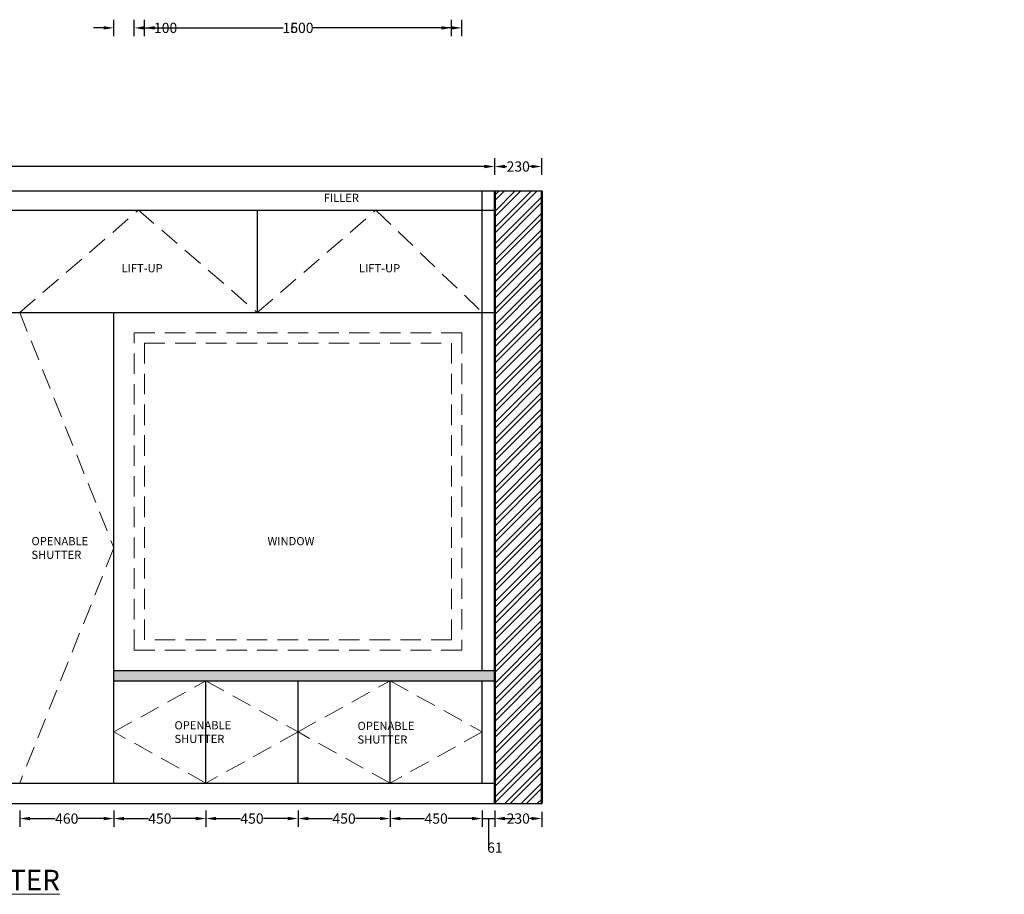
# Model space of a CAD drawing. Units: millimetres. Extents: x -472 to 16192, y -4730 to 4331.
# Tile 2 of 8: x 3049 to 7860, y -4730 to -455. Entities that reach past the tile are written whole.
import ezdxf

# ---------------------------------------------------------------- set-up
doc = ezdxf.new("R2010")
doc.units = ezdxf.units.MM
doc.header["$MEASUREMENT"] = 0
doc.linetypes.add('DASHED', pattern=[0.75, 0.5, -0.25])
for name, color, linetype, lineweight in [('A-ANNO-DIMS', 2, 'Continuous', 18), ('A-ANNO-TEXT', 6, 'Continuous', 18), ('A-ELEV', 7, 'Continuous', 25), ('A-ELEV-SWNG', 4, 'DASHED', 13), ('A-GLAZ', 4, 'DASHED', 18), ('A-WALL', 7, 'Continuous', 50), ('A-WALL-PATT', 8, 'Continuous', 13)]:
    doc.layers.add(name, color=color, linetype=linetype, lineweight=lineweight)
doc.styles.get("Standard").update_dxf_attribs({"font": 'arial.ttf'})
doc.dimstyles.get("Standard").update_dxf_attribs({"dimtxt": 50, "dimasz": 50, "dimexe": 40, "dimexo": 40, "dimgap": 0.09, "dimtad": 0, "dimtih": 1, "dimtoh": 1, "dimdec": 0, "dimzin": 0, "dimdsep": 46, "dimtxsty": 'Standard', "dimcen": 0.09, "dimclrd": 1, "dimclre": 3, "dimclrt": 6, "dimadec": 0, "dimazin": 0, "dimtfac": 1, "dimtdec": 0, "dimtofl": 0, "dimtmove": 0, "dimatfit": 3, "dimfxl": 40, "dimfxlon": 1, "dimtolj": 1, "dimtzin": 0, "dimarcsym": 0})

# ---------------------------------------------------------------- blocks, each defined once
blk = doc.blocks.new('*D17')
at = {"layer": 'A-ANNO-DIMS', "color": 0, "lineweight": -2, "transparency": 16777216}
for p, q in [((230, -1212.4), (230, -1132.4)), ((5370, -1212.4), (5370, -1132.4)), ((280, -1172.4), (2725.3, -1172.4)), ((5320, -1172.4), (2874.7, -1172.4))]:
    blk.add_line(p, q, dxfattribs=at)
at = {"layer": 'A-ANNO-DIMS', "color": 0, "transparency": 16777216}
for points in [[(280, -1164.1), (280, -1180.8), (230, -1172.4)], [(5320, -1164.1), (5320, -1180.8), (5370, -1172.4)]]:
    blk.add_solid(points, dxfattribs=at)
at = {"layer": 'Defpoints', "color": 0, "transparency": 16777216}
for p in [(5370, -1172.4), (230, -1290.9), (5370, -1290.9)]:
    blk.add_point(p, dxfattribs=at)
at = {"layer": 'A-ANNO-DIMS', "color": 0, "transparency": 16777216, "insert": (2800, -1172.4), "char_height": 50, "attachment_point": 5}
blk.add_mtext('\\A1;5140', dxfattribs=at)
blk = doc.blocks.new('*D18')
at = {"layer": 'A-ANNO-DIMS', "color": 0, "lineweight": -2, "transparency": 16777216}
for p, q in [((5370, -1212.4), (5370, -1132.4)), ((5600, -1212.4), (5600, -1132.4)), ((5420, -1172.4), (5429.3, -1172.4)), ((5550, -1172.4), (5540.7, -1172.4))]:
    blk.add_line(p, q, dxfattribs=at)
at = {"layer": 'A-ANNO-DIMS', "color": 0, "transparency": 16777216}
for points in [[(5420, -1164.1), (5420, -1180.8), (5370, -1172.4)], [(5550, -1164.1), (5550, -1180.8), (5600, -1172.4)]]:
    blk.add_solid(points, dxfattribs=at)
at = {"layer": 'Defpoints', "color": 0, "transparency": 16777216}
for p in [(5600, -1172.4), (5370, -1290.9), (5600, -1290.9)]:
    blk.add_point(p, dxfattribs=at)
at = {"layer": 'A-ANNO-DIMS', "color": 0, "transparency": 16777216, "insert": (5485, -1172.4), "char_height": 50, "attachment_point": 5}
blk.add_mtext('\\A1;230', dxfattribs=at)
blk = doc.blocks.new('*D34')
at = {"layer": 'A-ANNO-DIMS', "color": 0, "lineweight": -2, "transparency": 16777216}
for p, q in [((3049, -4319.4), (3049, -4399.4)), ((3509, -4319.4), (3509, -4399.4)), ((3099, -4359.4), (3222.8, -4359.4)), ((3459, -4359.4), (3335.2, -4359.4))]:
    blk.add_line(p, q, dxfattribs=at)
at = {"layer": 'A-ANNO-DIMS', "color": 0, "transparency": 16777216}
for points in [[(3099, -4351), (3099, -4367.7), (3049, -4359.4)], [(3459, -4351), (3459, -4367.7), (3509, -4359.4)]]:
    blk.add_solid(points, dxfattribs=at)
at = {"layer": 'Defpoints', "color": 0, "transparency": 16777216}
for p in [(3049, -4185.9), (3509, -4185.9), (3509, -4359.4)]:
    blk.add_point(p, dxfattribs=at)
at = {"layer": 'A-ANNO-DIMS', "color": 0, "transparency": 16777216, "insert": (3279, -4359.4), "char_height": 50, "attachment_point": 5}
blk.add_mtext('\\A1;460', dxfattribs=at)
blk = doc.blocks.new('*D35')
at = {"layer": 'A-ANNO-DIMS', "color": 0, "lineweight": -2, "transparency": 16777216}
for p, q in [((3509, -4319.4), (3509, -4399.4)), ((3959, -4319.4), (3959, -4399.4)), ((3559, -4359.4), (3677.8, -4359.4)), ((3909, -4359.4), (3790.2, -4359.4))]:
    blk.add_line(p, q, dxfattribs=at)
at = {"layer": 'A-ANNO-DIMS', "color": 0, "transparency": 16777216}
for points in [[(3559, -4351), (3559, -4367.7), (3509, -4359.4)], [(3909, -4351), (3909, -4367.7), (3959, -4359.4)]]:
    blk.add_solid(points, dxfattribs=at)
at = {"layer": 'Defpoints', "color": 0, "transparency": 16777216}
for p in [(3509, -4185.9), (3959, -4185.9), (3959, -4359.4)]:
    blk.add_point(p, dxfattribs=at)
at = {"layer": 'A-ANNO-DIMS', "color": 0, "transparency": 16777216, "insert": (3734, -4359.4), "char_height": 50, "attachment_point": 5}
blk.add_mtext('\\A1;450', dxfattribs=at)
blk = doc.blocks.new('*D36')
at = {"layer": 'A-ANNO-DIMS', "color": 0, "lineweight": -2, "transparency": 16777216}
for p, q in [((3959, -4319.4), (3959, -4399.4)), ((4409, -4319.4), (4409, -4399.4)), ((4009, -4359.4), (4127.8, -4359.4)), ((4359, -4359.4), (4240.2, -4359.4))]:
    blk.add_line(p, q, dxfattribs=at)
at = {"layer": 'A-ANNO-DIMS', "color": 0, "transparency": 16777216}
for points in [[(4009, -4351), (4009, -4367.7), (3959, -4359.4)], [(4359, -4351), (4359, -4367.7), (4409, -4359.4)]]:
    blk.add_solid(points, dxfattribs=at)
at = {"layer": 'Defpoints', "color": 0, "transparency": 16777216}
for p in [(3959, -4185.9), (4409, -4185.9), (4409, -4359.4)]:
    blk.add_point(p, dxfattribs=at)
at = {"layer": 'A-ANNO-DIMS', "color": 0, "transparency": 16777216, "insert": (4184, -4359.4), "char_height": 50, "attachment_point": 5}
blk.add_mtext('\\A1;450', dxfattribs=at)
blk = doc.blocks.new('*D37')
at = {"layer": 'A-ANNO-DIMS', "color": 0, "lineweight": -2, "transparency": 16777216}
for p, q in [((4409, -4319.4), (4409, -4399.4)), ((4859, -4319.4), (4859, -4399.4)), ((4459, -4359.4), (4577.8, -4359.4)), ((4809, -4359.4), (4690.2, -4359.4))]:
    blk.add_line(p, q, dxfattribs=at)
at = {"layer": 'A-ANNO-DIMS', "color": 0, "transparency": 16777216}
for points in [[(4459, -4351), (4459, -4367.7), (4409, -4359.4)], [(4809, -4351), (4809, -4367.7), (4859, -4359.4)]]:
    blk.add_solid(points, dxfattribs=at)
at = {"layer": 'Defpoints', "color": 0, "transparency": 16777216}
for p in [(4409, -4185.9), (4859, -4185.9), (4859, -4359.4)]:
    blk.add_point(p, dxfattribs=at)
at = {"layer": 'A-ANNO-DIMS', "color": 0, "transparency": 16777216, "insert": (4634, -4359.4), "char_height": 50, "attachment_point": 5}
blk.add_mtext('\\A1;450', dxfattribs=at)
blk = doc.blocks.new('*D38')
at = {"layer": 'A-ANNO-DIMS', "color": 0, "lineweight": -2, "transparency": 16777216}
for p, q in [((4859, -4319.4), (4859, -4399.4)), ((5309, -4319.4), (5309, -4399.4)), ((4909, -4359.4), (5027.8, -4359.4)), ((5259, -4359.4), (5140.2, -4359.4))]:
    blk.add_line(p, q, dxfattribs=at)
at = {"layer": 'A-ANNO-DIMS', "color": 0, "transparency": 16777216}
for points in [[(4909, -4351), (4909, -4367.7), (4859, -4359.4)], [(5259, -4351), (5259, -4367.7), (5309, -4359.4)]]:
    blk.add_solid(points, dxfattribs=at)
at = {"layer": 'Defpoints', "color": 0, "transparency": 16777216}
for p in [(4859, -4185.9), (5309, -4185.9), (5309, -4359.4)]:
    blk.add_point(p, dxfattribs=at)
at = {"layer": 'A-ANNO-DIMS', "color": 0, "transparency": 16777216, "insert": (5084, -4359.4), "char_height": 50, "attachment_point": 5}
blk.add_mtext('\\A1;450', dxfattribs=at)
blk = doc.blocks.new('*D39')
at = {"layer": 'A-ANNO-DIMS', "color": 0, "lineweight": -2, "transparency": 16777216}
for p, q in [((5309, -4319.4), (5309, -4399.4)), ((5370, -4319.4), (5370, -4399.4)), ((5259, -4359.4), (5209, -4359.4)), ((5309, -4359.4), (5370, -4359.4)), ((5339.5, -4359.4), (5339.5, -4501.5)), ((5420, -4359.4), (5470, -4359.4)), ((5339.5, -4501.5), (5339.7, -4501.5))]:
    blk.add_line(p, q, dxfattribs=at)
at = {"layer": 'A-ANNO-DIMS', "color": 0, "transparency": 16777216}
for points in [[(5259, -4351), (5259, -4367.7), (5309, -4359.4)], [(5420, -4351), (5420, -4367.7), (5370, -4359.4)]]:
    blk.add_solid(points, dxfattribs=at)
at = {"layer": 'Defpoints', "color": 0, "transparency": 16777216}
for p in [(5309, -4185.9), (5370, -4185.9), (5370, -4359.4)]:
    blk.add_point(p, dxfattribs=at)
at = {"layer": 'A-ANNO-DIMS', "color": 0, "transparency": 16777216, "insert": (5370.9, -4501.5), "char_height": 50, "attachment_point": 5}
blk.add_mtext('\\A1;61', dxfattribs=at)
blk = doc.blocks.new('*D40')
at = {"layer": 'A-ANNO-DIMS', "color": 0, "lineweight": -2, "transparency": 16777216}
for p, q in [((5370, -4319.4), (5370, -4399.4)), ((5600, -4325.9), (5600, -4399.4)), ((5420, -4359.4), (5429.3, -4359.4)), ((5550, -4359.4), (5540.7, -4359.4))]:
    blk.add_line(p, q, dxfattribs=at)
at = {"layer": 'A-ANNO-DIMS', "color": 0, "transparency": 16777216}
for points in [[(5420, -4351), (5420, -4367.7), (5370, -4359.4)], [(5550, -4351), (5550, -4367.7), (5600, -4359.4)]]:
    blk.add_solid(points, dxfattribs=at)
at = {"layer": 'Defpoints', "color": 0, "transparency": 16777216}
for p in [(5370, -4185.9), (5600, -4285.9), (5600, -4359.4)]:
    blk.add_point(p, dxfattribs=at)
at = {"layer": 'A-ANNO-DIMS', "color": 0, "transparency": 16777216, "insert": (5485, -4359.4), "char_height": 50, "attachment_point": 5}
blk.add_mtext('\\A1;230', dxfattribs=at)
blk = doc.blocks.new('*D97')
at = {"layer": 'A-ANNO-DIMS', "color": 3, "lineweight": -2, "transparency": 16777216}
for p, q in [((3509, -534.9), (3509, -454.9)), ((3609, -534.9), (3609, -454.9))]:
    blk.add_line(p, q, dxfattribs=at)
at = {"layer": 'A-ANNO-DIMS', "color": 1, "lineweight": -2, "transparency": 16777216}
for p, q in [((3459, -494.9), (3409, -494.9)), ((3659, -494.9), (3709, -494.9))]:
    blk.add_line(p, q, dxfattribs=at)
at = {"layer": 'A-ANNO-DIMS', "color": 1, "transparency": 16777216}
for points in [[(3459, -486.6), (3459, -503.2), (3509, -494.9)], [(3659, -486.6), (3659, -503.2), (3609, -494.9)]]:
    blk.add_solid(points, dxfattribs=at)
at = {"layer": 'Defpoints', "color": 0, "transparency": 16777216}
for p in [(3609, -494.9), (3509, -1885.9), (3609, -1985.9)]:
    blk.add_point(p, dxfattribs=at)
at = {"layer": 'A-ANNO-DIMS', "color": 6, "transparency": 16777216, "insert": (3761.9, -494.9), "char_height": 50, "attachment_point": 5}
blk.add_mtext('\\A1;100', dxfattribs=at)
blk = doc.blocks.new('*D98')
at = {"layer": 'A-ANNO-DIMS', "color": 3, "lineweight": -2, "transparency": 16777216}
for p, q in [((3609, -534.9), (3609, -454.9)), ((5209, -534.9), (5209, -454.9))]:
    blk.add_line(p, q, dxfattribs=at)
at = {"layer": 'A-ANNO-DIMS', "color": 1, "lineweight": -2, "transparency": 16777216}
for p, q in [((3659, -494.9), (4336.7, -494.9)), ((5159, -494.9), (4481.3, -494.9))]:
    blk.add_line(p, q, dxfattribs=at)
at = {"layer": 'A-ANNO-DIMS', "color": 1, "transparency": 16777216}
for points in [[(3659, -486.6), (3659, -503.2), (3609, -494.9)], [(5159, -486.6), (5159, -503.2), (5209, -494.9)]]:
    blk.add_solid(points, dxfattribs=at)
at = {"layer": 'Defpoints', "color": 0, "transparency": 16777216}
for p in [(5209, -494.9), (3609, -1985.9), (5209, -1985.9)]:
    blk.add_point(p, dxfattribs=at)
at = {"layer": 'A-ANNO-DIMS', "color": 6, "transparency": 16777216, "insert": (4409, -494.9), "char_height": 50, "attachment_point": 5}
blk.add_mtext('\\A1;1600', dxfattribs=at)
blk = doc.blocks.new('*D99')
at = {"layer": 'A-ANNO-DIMS', "color": 3, "lineweight": -2, "transparency": 16777216}
for p, q in [((3659, -534.9), (3659, -454.9)), ((5159, -534.9), (5159, -454.9))]:
    blk.add_line(p, q, dxfattribs=at)
at = {"layer": 'A-ANNO-DIMS', "color": 1, "lineweight": -2, "transparency": 16777216}
for p, q in [((3709, -494.9), (4336.7, -494.9)), ((5109, -494.9), (4481.3, -494.9))]:
    blk.add_line(p, q, dxfattribs=at)
at = {"layer": 'A-ANNO-DIMS', "color": 1, "transparency": 16777216}
for points in [[(3709, -486.6), (3709, -503.2), (3659, -494.9)], [(5109, -486.6), (5109, -503.2), (5159, -494.9)]]:
    blk.add_solid(points, dxfattribs=at)
at = {"layer": 'Defpoints', "color": 0, "transparency": 16777216}
for p in [(5159, -494.9), (3659, -2035.9), (5159, -2035.9)]:
    blk.add_point(p, dxfattribs=at)
at = {"layer": 'A-ANNO-DIMS', "color": 6, "transparency": 16777216, "insert": (4409, -494.9), "char_height": 50, "attachment_point": 5}
blk.add_mtext('\\A1;1500', dxfattribs=at)
blk = doc.blocks.new('*D100')
at = {"layer": 'A-ANNO-DIMS', "color": 1, "lineweight": -2, "transparency": 16777216}
for p, q in [((16116.7, -1835.9), (16116.7, -1785.9)), ((16116.7, -2035.9), (16116.7, -2085.9))]:
    blk.add_line(p, q, dxfattribs=at)
at = {"layer": 'A-ANNO-DIMS', "color": 3, "lineweight": -2, "transparency": 16777216}
for p, q in [((16076.7, -1885.9), (16156.7, -1885.9)), ((16076.7, -1985.9), (16156.7, -1985.9))]:
    blk.add_line(p, q, dxfattribs=at)
at = {"layer": 'A-ANNO-DIMS', "color": 1, "transparency": 16777216}
for points in [[(16108.3, -1835.9), (16125, -1835.9), (16116.7, -1885.9)], [(16108.3, -2035.9), (16125, -2035.9), (16116.7, -1985.9)]]:
    blk.add_solid(points, dxfattribs=at)
at = {"layer": 'Defpoints', "color": 0, "transparency": 16777216}
for p in [(5309, -1885.9), (5209, -1985.9), (16116.7, -1985.9)]:
    blk.add_point(p, dxfattribs=at)
at = {"layer": 'A-ANNO-DIMS', "color": 6, "transparency": 16777216, "insert": (16116.7, -1935.9), "char_height": 50, "attachment_point": 5}
blk.add_mtext('\\A1;100', dxfattribs=at)
blk = doc.blocks.new('*D101')
at = {"layer": 'A-ANNO-DIMS', "color": 3, "lineweight": -2, "transparency": 16777216}
for p, q in [((16076.7, -1985.9), (16156.7, -1985.9)), ((16076.7, -3535.9), (16156.7, -3535.9))]:
    blk.add_line(p, q, dxfattribs=at)
at = {"layer": 'A-ANNO-DIMS', "color": 1, "lineweight": -2, "transparency": 16777216}
for p, q in [((16116.7, -2035.9), (16116.7, -2735.3)), ((16116.7, -3485.9), (16116.7, -2786.5))]:
    blk.add_line(p, q, dxfattribs=at)
at = {"layer": 'A-ANNO-DIMS', "color": 1, "transparency": 16777216}
for points in [[(16108.3, -2035.9), (16125, -2035.9), (16116.7, -1985.9)], [(16108.3, -3485.9), (16125, -3485.9), (16116.7, -3535.9)]]:
    blk.add_solid(points, dxfattribs=at)
at = {"layer": 'Defpoints', "color": 0, "transparency": 16777216}
for p in [(5209, -1985.9), (5209, -3535.9), (16116.7, -3535.9)]:
    blk.add_point(p, dxfattribs=at)
at = {"layer": 'A-ANNO-DIMS', "color": 6, "transparency": 16777216, "insert": (16116.7, -2760.9), "char_height": 50, "attachment_point": 5}
blk.add_mtext('\\A1;1550', dxfattribs=at)
blk = doc.blocks.new('*D102')
at = {"layer": 'A-ANNO-DIMS', "color": 3, "lineweight": -2, "transparency": 16777216}
for p, q in [((16076.7, -2035.9), (16156.7, -2035.9)), ((16076.7, -3485.9), (16156.7, -3485.9))]:
    blk.add_line(p, q, dxfattribs=at)
at = {"layer": 'A-ANNO-DIMS', "color": 1, "lineweight": -2, "transparency": 16777216}
for p, q in [((16116.7, -2085.9), (16116.7, -2735.3)), ((16116.7, -3435.9), (16116.7, -2786.5))]:
    blk.add_line(p, q, dxfattribs=at)
at = {"layer": 'A-ANNO-DIMS', "color": 1, "transparency": 16777216}
for points in [[(16108.3, -2085.9), (16125, -2085.9), (16116.7, -2035.9)], [(16108.3, -3435.9), (16125, -3435.9), (16116.7, -3485.9)]]:
    blk.add_solid(points, dxfattribs=at)
at = {"layer": 'Defpoints', "color": 0, "transparency": 16777216}
for p in [(5159, -2035.9), (5159, -3485.9), (16116.7, -3485.9)]:
    blk.add_point(p, dxfattribs=at)
at = {"layer": 'A-ANNO-DIMS', "color": 6, "transparency": 16777216, "insert": (16116.7, -2760.9), "char_height": 50, "attachment_point": 5}
blk.add_mtext('\\A1;1450', dxfattribs=at)
blk = doc.blocks.new('*D103')
at = {"layer": 'A-ANNO-DIMS', "color": 1, "lineweight": -2, "transparency": 16777216}
for p, q in [((16116.7, -3485.9), (16116.7, -3435.9)), ((16116.7, -3685.9), (16116.7, -3735.9))]:
    blk.add_line(p, q, dxfattribs=at)
at = {"layer": 'A-ANNO-DIMS', "color": 3, "lineweight": -2, "transparency": 16777216}
for p, q in [((16076.7, -3535.9), (16156.7, -3535.9)), ((16076.7, -3635.9), (16156.7, -3635.9))]:
    blk.add_line(p, q, dxfattribs=at)
at = {"layer": 'A-ANNO-DIMS', "color": 1, "transparency": 16777216}
for points in [[(16108.3, -3485.9), (16125, -3485.9), (16116.7, -3535.9)], [(16108.3, -3685.9), (16125, -3685.9), (16116.7, -3635.9)]]:
    blk.add_solid(points, dxfattribs=at)
at = {"layer": 'Defpoints', "color": 0, "transparency": 16777216}
for p in [(5209, -3535.9), (5309, -3635.9), (16116.7, -3635.9)]:
    blk.add_point(p, dxfattribs=at)
at = {"layer": 'A-ANNO-DIMS', "color": 6, "transparency": 16777216, "insert": (16116.7, -3585.9), "char_height": 50, "attachment_point": 5}
blk.add_mtext('\\A1;100', dxfattribs=at)
blk = doc.blocks.new('*D104')
at = {"layer": 'A-ANNO-DIMS', "color": 1, "lineweight": -2, "transparency": 16777216}
for p, q in [((16116.7, -3585.9), (16116.7, -3535.9)), ((16116.7, -3735.9), (16116.7, -3785.9)), ((16116.7, -3785.9), (16066.7, -3785.9))]:
    blk.add_line(p, q, dxfattribs=at)
at = {"layer": 'A-ANNO-DIMS', "color": 3, "lineweight": -2, "transparency": 16777216}
for p, q in [((16076.7, -3635.9), (16156.7, -3635.9)), ((16076.7, -3685.9), (16156.7, -3685.9))]:
    blk.add_line(p, q, dxfattribs=at)
at = {"layer": 'A-ANNO-DIMS', "color": 1, "transparency": 16777216}
for points in [[(16108.3, -3585.9), (16125, -3585.9), (16116.7, -3635.9)], [(16108.3, -3735.9), (16125, -3735.9), (16116.7, -3685.9)]]:
    blk.add_solid(points, dxfattribs=at)
at = {"layer": 'Defpoints', "color": 0, "transparency": 16777216}
for p in [(5309, -3635.9), (5309, -3685.9), (16116.7, -3685.9)]:
    blk.add_point(p, dxfattribs=at)
at = {"layer": 'A-ANNO-DIMS', "color": 6, "transparency": 16777216, "insert": (16030.8, -3785.9), "char_height": 50, "attachment_point": 5}
blk.add_mtext('\\A1;50', dxfattribs=at)

msp = doc.modelspace()

# ---------------------------------------------------------------- hatches: boundary and pattern name
at = {"layer": 'A-GLAZ'}
h = msp.add_hatch(color=256, dxfattribs=at)
h.dxf.hatch_style = 1
h.paths.add_polyline_path([(5370, -3635.9), (3509, -3635.9), (3509, -3685.9), (5309, -3685.9), (5370, -3685.9)])
at = {"layer": 'A-WALL-PATT'}
h = msp.add_hatch(dxfattribs=at)
h.set_pattern_fill('ANSI32', color=256, scale=150)
h.paths.add_polyline_path([(9720.7, -1290.9), (9720.7, -4285.9), (9950.7, -4285.9), (9950.7, -4185.9), (9950.7, -1885.9), (9950.7, -1290.9)])
h.paths.add_polyline_path([(5370, -4285.9), (5600, -4285.9), (5600, -1290.9), (5370, -1290.9)])
h.paths.add_polyline_path([(15320.7, -1290.9), (15090.7, -1290.9), (15090.7, -4285.9), (15320.7, -4285.9)])
h.paths.add_polyline_path([(0, -4285.9), (230, -4285.9), (230, -4185.9), (230, -1885.9), (230, -1290.9), (0, -1290.9)])

# ---------------------------------------------------------------- linework, layer by layer
at = {"layer": 'A-ELEV'}
for p, q in [((0, -1290.9), (5600, -1290.9)), ((5309, -3635.9), (5309, -1290.9)), ((230, -1385.9), (3049, -1385.9)), ((3049, -1385.9), (5370, -1385.9)), ((4209.5, -1385.9), (4209.5, -1885.9)), ((230, -1885.9), (5370, -1885.9)), ((3509, -3685.9), (3509, -1885.9)), ((3509, -3635.9), (5370, -3635.9)), ((3509, -4185.9), (3509, -3685.9)), ((3509, -3685.9), (5370, -3685.9)), ((3959, -4185.9), (3959, -3685.9)), ((4409, -4185.9), (4409, -3685.9)), ((4859, -4185.9), (4859, -3685.9)), ((5309, -4185.9), (5309, -3685.9)), ((230, -4185.9), (3509, -4185.9)), ((3509, -4185.9), (5370, -4185.9)), ((0, -4285.9), (5600, -4285.9))]:
    msp.add_line(p, q, dxfattribs=at)
at = {"layer": 'A-ELEV-SWNG', "ltscale": 200}
for p, q in [((3049, -1885.9), (3629.3, -1385.9)), ((3629.3, -1385.9), (4209.5, -1885.9)), ((4209.5, -1885.9), (4789.8, -1385.9)), ((4789.8, -1385.9), (5309, -1885.9)), ((3049, -1885.9), (3509, -3035.9)), ((3509, -3035.9), (3049, -4185.9)), ((3509, -3935.9), (3959, -3685.9)), ((3959, -3685.9), (4409, -3935.9)), ((4409, -3935.9), (4859, -3685.9)), ((4859, -3685.9), (5309, -3935.9)), ((3959, -4185.9), (3509, -3935.9)), ((4409, -3935.9), (3959, -4185.9)), ((4859, -4185.9), (4409, -3935.9)), ((5309, -3935.9), (4859, -4185.9))]:
    msp.add_line(p, q, dxfattribs=at)
at = {"layer": 'A-GLAZ', "ltscale": 200}
for points in [[(3609, -1985.9), (5209, -1985.9), (5209, -3535.9), (3609, -3535.9)], [(3659, -2035.9), (5159, -2035.9), (5159, -3485.9), (3659, -3485.9)]]:
    msp.add_lwpolyline(points, close=True, dxfattribs=at)
at = {"layer": 'A-WALL'}
for p, q in [((5370, -4285.9), (5370, -1290.9)), ((5600, -4285.9), (5600, -1290.9))]:
    msp.add_line(p, q, dxfattribs=at)

# ---------------------------------------------------------------- texts
at = {"layer": 'A-ANNO-TEXT', "attachment_point": 1}
for s, width, insert, char_height in [('FILLER', 327.678, (4534.8, -1305.7), 40), ('LIFT-UP', 327.678, (3546.4, -1649.6), 40), ('LIFT-UP', 327.678, (4706.9, -1649.6), 40), ('OPENABLE \\PSHUTTER', 327.678, (3106.4, -2983.4), 40), ('WINDOW', 327.678, (4259.7, -2983.4), 40), ('OPENABLE \\PSHUTTER', 327.678, (3805.3, -3883.4), 40), ('OPENABLE \\PSHUTTER', 327.678, (4699.7, -3886.4), 40), ('{\\fArial|b1|i0|c0|p34;\\LELEVATION WITH SHUTTER}', 3435.915, (1516.3, -4609.6), 100)]:
    msp.add_mtext_dynamic_manual_height_columns(s, width=width, gutter_width=1, heights=[0], dxfattribs=dict(at, insert=insert, char_height=char_height))

# ---------------------------------------------------------------- dimensions: what is measured, and where the dimension line sits
at = {"layer": 'A-ANNO-DIMS'}
for base, p1, p2, override, picture, middle in [((3609, -494.9), (3509, -1885.9), (3609, -1985.9), {"dimdec": 0, "dimlfac": 1, "dimrnd": 0, "dimzin": 0, "dimdsep": 46, "dimlunit": 2}, '*D97', (3761.9, -494.9)), ((5209, -494.9), (3609, -1985.9), (5209, -1985.9), {"dimdec": 0, "dimlfac": 1, "dimrnd": 0, "dimzin": 0, "dimdsep": 46, "dimlunit": 2}, '*D98', (4409, -494.9)), ((5159, -494.9), (3659, -2035.9), (5159, -2035.9), {"dimdec": 0, "dimlfac": 1, "dimrnd": 0, "dimzin": 0, "dimdsep": 46, "dimlunit": 2}, '*D99', (4409, -494.9)), ((5370, -1172.4), (230, -1290.9), (5370, -1290.9), {"dimclrd": 0, "dimclre": 0, "dimclrt": 0}, '*D17', (2800, -1172.4)), ((5600, -1172.4), (5370, -1290.9), (5600, -1290.9), {"dimclrd": 0, "dimclre": 0, "dimclrt": 0}, '*D18', (5485, -1172.4)), ((3509, -4359.4), (3049, -4185.9), (3509, -4185.9), {"dimclrd": 0, "dimclre": 0, "dimclrt": 0, "dimtmove": 1}, '*D34', (3279, -4359.4)), ((3959, -4359.4), (3509, -4185.9), (3959, -4185.9), {"dimclrd": 0, "dimclre": 0, "dimclrt": 0, "dimtmove": 1}, '*D35', (3734, -4359.4)), ((4409, -4359.4), (3959, -4185.9), (4409, -4185.9), {"dimclrd": 0, "dimclre": 0, "dimclrt": 0, "dimtmove": 1}, '*D36', (4184, -4359.4)), ((4859, -4359.4), (4409, -4185.9), (4859, -4185.9), {"dimclrd": 0, "dimclre": 0, "dimclrt": 0, "dimtmove": 1}, '*D37', (4634, -4359.4)), ((5309, -4359.4), (4859, -4185.9), (5309, -4185.9), {"dimclrd": 0, "dimclre": 0, "dimclrt": 0, "dimtmove": 1}, '*D38', (5084, -4359.4)), ((5370, -4359.4), (5309, -4185.9), (5370, -4185.9), {"dimclrd": 0, "dimclre": 0, "dimclrt": 0, "dimtmove": 1}, '*D39', (5339.8, -4501.5)), ((5600, -4359.4), (5370, -4185.9), (5600, -4285.9), {"dimclrd": 0, "dimclre": 0, "dimclrt": 0, "dimtmove": 1}, '*D40', (5485, -4359.4))]:
    dim = msp.add_linear_dim(base=base, p1=p1, p2=p2, dimstyle='Standard', override=override, dxfattribs=at)
    dim.commit()
    dim.dimension.update_dxf_attribs({"geometry": picture, "text_midpoint": middle})
for base, p1, p2, picture, middle in [((16116.7, -1985.9), (5309, -1885.9), (5209, -1985.9), '*D100', (16116.7, -1935.9)), ((16116.7, -3535.9), (5209, -1985.9), (5209, -3535.9), '*D101', (16116.7, -2760.9)), ((16116.7, -3485.9), (5159, -2035.9), (5159, -3485.9), '*D102', (16116.7, -2760.9)), ((16116.7, -3635.9), (5209, -3535.9), (5309, -3635.9), '*D103', (16116.7, -3585.9)), ((16116.7, -3685.9), (5309, -3635.9), (5309, -3685.9), '*D104', (16030.8, -3785.9))]:
    dim = msp.add_linear_dim(base=base, p1=p1, p2=p2, angle=90, dimstyle='Standard', override={"dimdec": 0, "dimlfac": 1, "dimrnd": 0, "dimzin": 0, "dimdsep": 46, "dimlunit": 2}, dxfattribs=at)
    dim.commit()
    dim.dimension.update_dxf_attribs({"geometry": picture, "text_midpoint": middle})

doc.saveas('drawing.dxf')
